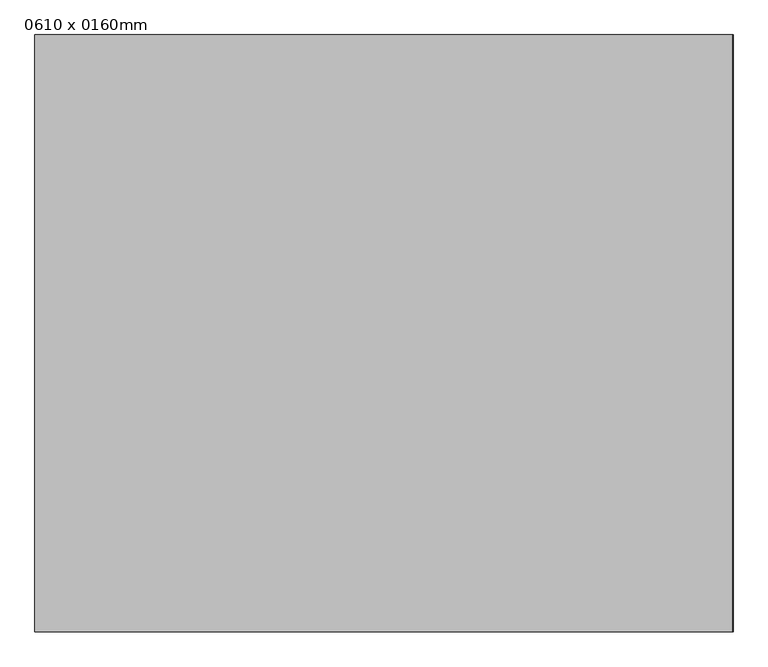
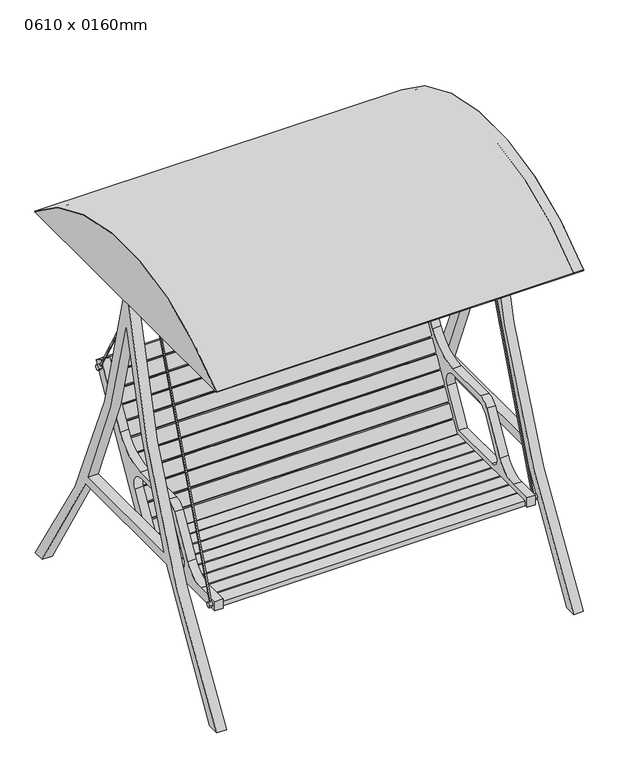
"""IFC4 building model written with IfcOpenShell, lengths in millimetres: furniture geometry, 0610 x 0160mm."""

from ifc_helpers import new_model, si_unit, point, frame, frame_2d, origin, place, context, project, spatial, polyline, circle_curve, trimmed, segment, composite_curve, outline, extrude, source, transform, mapped, element, save


def furniture_0610_x_0160mm_a8fad5e2(model_context):
    return source(origin(), model_context, "Body", "SweptSolid", [
        extrude(outline(composite_curve([segment(trimmed(circle_curve(frame_2d((4189.9023331, 1950.2809332)), 3303.1244251), [point((933.45, 1396.9734505))], [point((1524.0, 0.0))], True, "CARTESIAN"), True, "CONTINUOUS"), segment(polyline([(1524.0, 0.0), (1476.936255, 0.0)]), True, "CONTINUOUS"), segment(trimmed(circle_curve(frame_2d((4189.9023331, 1950.2809332)), 3341.2244251), [point((1476.936255, 0.0))], [point((1186.3373595, 486.5944542))], False, "CARTESIAN"), True, "CONTINUOUS"), segment(polyline([(1186.3373595, 486.5944542), (642.4626405, 486.5944542)]), True, "CONTINUOUS"), segment(trimmed(circle_curve(frame_2d((-2361.1023331, 1950.2809332)), 3341.2244251), [point((642.4626405, 486.5944542))], [point((351.863745, 0.0))], False, "CARTESIAN"), True, "CONTINUOUS"), segment(polyline([(351.863745, 0.0), (304.8, 0.0)]), True, "CONTINUOUS"), segment(trimmed(circle_curve(frame_2d((-2361.1023331, 1950.2809332)), 3303.1244251), [point((304.8, 0.0))], [point((895.35, 1396.9734505))], True, "CARTESIAN"), True, "CONTINUOUS"), segment(polyline([(895.35, 1396.9734505), (895.35, 1524.0), (914.4, 1524.0), (933.45, 1524.0), (933.45, 1396.9734505)]), True, "CONTINUOUS")], self_intersect=False), holes=[composite_curve([segment(polyline([(660.7321842, 524.6944542), (1168.0678158, 524.6944542)]), True, "CONTINUOUS"), segment(trimmed(circle_curve(frame_2d((4189.9023331, 1950.2809332)), 3341.2244251), [point((1168.0678158, 524.6944542))], [point((914.4, 1290.8378915))], False, "CARTESIAN"), True, "CONTINUOUS"), segment(trimmed(circle_curve(frame_2d((-2361.1023331, 1950.2809332)), 3341.2244251), [point((914.4, 1290.8378915))], [point((660.7321842, 524.6944542))], False, "CARTESIAN"), True, "CONTINUOUS")], self_intersect=False)]), frame((-272.362745, 0.0, 0.0), z_axis=(1.0, 0.0, 0.0), x_axis=(0.0, 1.0, 0.0)), (0.0, 0.0, 1.0), 38.1),
        extrude(outline(composite_curve([segment(trimmed(circle_curve(frame_2d((4189.9023331, 1950.2809332)), 3303.1244251), [point((933.45, 1396.9734505))], [point((1524.0, 0.0))], True, "CARTESIAN"), True, "CONTINUOUS"), segment(polyline([(1524.0, 0.0), (1476.936255, 0.0)]), True, "CONTINUOUS"), segment(trimmed(circle_curve(frame_2d((4189.9023331, 1950.2809332)), 3341.2244251), [point((1476.936255, 0.0))], [point((1186.3373595, 486.5944542))], False, "CARTESIAN"), True, "CONTINUOUS"), segment(polyline([(1186.3373595, 486.5944542), (642.4626405, 486.5944542)]), True, "CONTINUOUS"), segment(trimmed(circle_curve(frame_2d((-2361.1023331, 1950.2809332)), 3341.2244251), [point((642.4626405, 486.5944542))], [point((351.863745, 0.0))], False, "CARTESIAN"), True, "CONTINUOUS"), segment(polyline([(351.863745, 0.0), (304.8, 0.0)]), True, "CONTINUOUS"), segment(trimmed(circle_curve(frame_2d((-2361.1023331, 1950.2809332)), 3303.1244251), [point((304.8, 0.0))], [point((895.35, 1396.9734505))], True, "CARTESIAN"), True, "CONTINUOUS"), segment(polyline([(895.35, 1396.9734505), (895.35, 1524.0), (914.4, 1524.0), (933.45, 1524.0), (933.45, 1396.9734505)]), True, "CONTINUOUS")], self_intersect=False), holes=[composite_curve([segment(polyline([(660.7321842, 524.6944542), (1168.0678158, 524.6944542)]), True, "CONTINUOUS"), segment(trimmed(circle_curve(frame_2d((4189.9023331, 1950.2809332)), 3341.2244251), [point((1168.0678158, 524.6944542))], [point((914.4, 1290.8378915))], False, "CARTESIAN"), True, "CONTINUOUS"), segment(trimmed(circle_curve(frame_2d((-2361.1023331, 1950.2809332)), 3341.2244251), [point((914.4, 1290.8378915))], [point((660.7321842, 524.6944542))], False, "CARTESIAN"), True, "CONTINUOUS")], self_intersect=False)]), frame((1111.937255, 0.0, 0.0), z_axis=(1.0, 0.0, 0.0), x_axis=(0.0, 1.0, 0.0)), (0.0, 0.0, 1.0), 38.1),
        extrude(outline(polyline([(1111.937255, 933.45), (1111.937255, 895.35), (-234.262745, 895.35), (-234.262745, 933.45), (1111.937255, 933.45)])), frame((0.0, 0.0, 1484.1023899), z_axis=(0.0, 0.0, 1.0), x_axis=(1.0, 0.0, 0.0)), (0.0, 0.0, 1.0), 39.8976101),
        extrude(outline(composite_curve([segment(trimmed(circle_curve(frame_2d((914.4, 699.3747703)), 926.421113), [point((304.8, 1396.9734505))], [point((1524.0, 1396.9734505))], False, "CARTESIAN"), True, "CONTINUOUS"), segment(polyline([(1524.0, 1396.9734505), (304.8, 1396.9734505)]), True, "CONTINUOUS")], self_intersect=False), holes=[composite_curve([segment(polyline([(376.708681, 1422.3734505), (1452.091319, 1422.3734505)]), True, "CONTINUOUS"), segment(trimmed(circle_curve(frame_2d((914.4, 699.3747703)), 901.021113), [point((1452.091319, 1422.3734505))], [point((376.708681, 1422.3734505))], True, "CARTESIAN"), True, "CONTINUOUS")], self_intersect=False)]), frame((-272.362745, 0.0, 0.0), z_axis=(1.0, 0.0, 0.0), x_axis=(0.0, 1.0, 0.0)), (0.0, 0.0, 1.0), 38.1),
        extrude(outline(composite_curve([segment(trimmed(circle_curve(frame_2d((914.4, 699.3747703)), 926.421113), [point((304.8, 1396.9734505))], [point((1524.0, 1396.9734505))], False, "CARTESIAN"), True, "CONTINUOUS"), segment(polyline([(1524.0, 1396.9734505), (304.8, 1396.9734505)]), True, "CONTINUOUS")], self_intersect=False), holes=[composite_curve([segment(polyline([(376.708681, 1422.3734505), (1452.091319, 1422.3734505)]), True, "CONTINUOUS"), segment(trimmed(circle_curve(frame_2d((914.4, 699.3747703)), 901.021113), [point((1452.091319, 1422.3734505))], [point((376.708681, 1422.3734505))], True, "CARTESIAN"), True, "CONTINUOUS")], self_intersect=False)]), frame((1111.937255, 0.0, 0.0), z_axis=(1.0, 0.0, 0.0), x_axis=(0.0, 1.0, 0.0)), (0.0, 0.0, 1.0), 38.1),
        extrude(outline(composite_curve([segment(trimmed(circle_curve(frame_2d((914.4, 699.3747703)), 926.421113), [point((304.8, 1396.9734505))], [point((1524.0, 1396.9734505))], False, "CARTESIAN"), True, "CONTINUOUS"), segment(polyline([(1524.0, 1396.9734505), (304.8, 1396.9734505)]), True, "CONTINUOUS")], self_intersect=False)), frame((-273.952745, 0.0, 0.0), z_axis=(1.0, 0.0, 0.0), x_axis=(0.0, 1.0, 0.0)), (0.0, 0.0, 1.0), 1.59),
        extrude(outline(composite_curve([segment(trimmed(circle_curve(frame_2d((914.4, 699.3747703)), 926.421113), [point((304.8, 1396.9734505))], [point((1524.0, 1396.9734505))], False, "CARTESIAN"), True, "CONTINUOUS"), segment(polyline([(1524.0, 1396.9734505), (304.8, 1396.9734505)]), True, "CONTINUOUS")], self_intersect=False)), frame((1150.037255, 0.0, 0.0), z_axis=(1.0, 0.0, 0.0), x_axis=(0.0, 1.0, 0.0)), (0.0, 0.0, 1.0), 1.59),
        extrude(outline(composite_curve([segment(trimmed(circle_curve(frame_2d((914.4, 699.3747703)), 926.421113), [point((1524.0, 1396.9734505))], [point((304.8, 1396.9734505))], True, "CARTESIAN"), True, "CONTINUOUS"), segment(polyline([(304.8, 1396.9734505), (304.8, 1399.0836139)]), True, "CONTINUOUS"), segment(trimmed(circle_curve(frame_2d((914.4, 699.3747703)), 928.011113), [point((304.8, 1399.0836139))], [point((1524.0, 1399.0836139))], False, "CARTESIAN"), True, "CONTINUOUS"), segment(polyline([(1524.0, 1399.0836139), (1524.0, 1396.9734505)]), True, "CONTINUOUS")], self_intersect=False)), frame((-273.952745, 0.0, 0.0), z_axis=(1.0, 0.0, 0.0), x_axis=(0.0, 1.0, 0.0)), (0.0, 0.0, 1.0), 1423.99),
        extrude(outline(composite_curve([segment(trimmed(circle_curve(frame_2d((563.6419667, 511.4)), 105.0), [point((563.6419667, 406.4))], [point((654.5746341, 458.9))], True, "CARTESIAN"), True, "CONTINUOUS"), segment(polyline([(654.5746341, 458.9), (741.8122598, 610.0)]), True, "CONTINUOUS"), segment(trimmed(circle_curve(frame_2d((785.11353, 585.0)), 50.0), [point((741.8122598, 610.0))], [point((785.11353, 635.0))], False, "CARTESIAN"), True, "CONTINUOUS"), segment(polyline([(785.11353, 635.0), (968.6699734, 635.0)]), True, "CONTINUOUS"), segment(trimmed(circle_curve(frame_2d((968.6699734, 795.0)), 160.0), [point((968.6699734, 635.0))], [point((1107.2340381, 715.0))], True, "CARTESIAN"), True, "CONTINUOUS"), segment(polyline([(1107.2340381, 715.0), (1233.863745, 934.3290861), (1266.8593129, 915.2790861), (951.0607902, 368.3), (471.863745, 368.3), (471.863745, 406.4), (563.6419667, 406.4)]), True, "CONTINUOUS")], self_intersect=False), holes=[composite_curve([segment(trimmed(circle_curve(frame_2d((807.1413638, 546.8466726)), 62.7533274), [point((807.1413638, 609.6))], [point((752.7953881, 578.2233363))], True, "CARTESIAN"), True, "CONTINUOUS"), segment(polyline([(752.7953881, 578.2233363), (679.5739008, 451.4)]), True, "CONTINUOUS"), segment(trimmed(circle_curve(frame_2d((705.5546629, 436.4)), 30.0), [point((679.5739008, 451.4))], [point((705.5546629, 406.4))], True, "CARTESIAN"), True, "CONTINUOUS"), segment(polyline([(705.5546629, 406.4), (929.063745, 406.4), (1007.4101765, 542.1)]), True, "CONTINUOUS"), segment(trimmed(circle_curve(frame_2d((968.4390333, 564.6)), 45.0), [point((1007.4101765, 542.1))], [point((968.4390333, 609.6))], True, "CARTESIAN"), True, "CONTINUOUS"), segment(polyline([(968.4390333, 609.6), (807.1413638, 609.6)]), True, "CONTINUOUS")], self_intersect=False)]), frame((-184.03019, 0.0, 0.0), z_axis=(1.0, 0.0, 0.0), x_axis=(0.0, 1.0, 0.0)), (0.0, 0.0, 1.0), 32.5713093),
        extrude(outline(composite_curve([segment(trimmed(circle_curve(frame_2d((563.6419667, 511.4)), 105.0), [point((563.6419667, 406.4))], [point((654.5746341, 458.9))], True, "CARTESIAN"), True, "CONTINUOUS"), segment(polyline([(654.5746341, 458.9), (741.8122598, 610.0)]), True, "CONTINUOUS"), segment(trimmed(circle_curve(frame_2d((785.11353, 585.0)), 50.0), [point((741.8122598, 610.0))], [point((785.11353, 635.0))], False, "CARTESIAN"), True, "CONTINUOUS"), segment(polyline([(785.11353, 635.0), (968.6699734, 635.0)]), True, "CONTINUOUS"), segment(trimmed(circle_curve(frame_2d((968.6699734, 795.0)), 160.0), [point((968.6699734, 635.0))], [point((1107.2340381, 715.0))], True, "CARTESIAN"), True, "CONTINUOUS"), segment(polyline([(1107.2340381, 715.0), (1233.863745, 934.3290861), (1266.8593129, 915.2790861), (951.0607902, 368.3), (471.863745, 368.3), (471.863745, 406.4), (563.6419667, 406.4)]), True, "CONTINUOUS")], self_intersect=False), holes=[composite_curve([segment(trimmed(circle_curve(frame_2d((807.1413638, 546.8466726)), 62.7533274), [point((807.1413638, 609.6))], [point((752.7953881, 578.2233363))], True, "CARTESIAN"), True, "CONTINUOUS"), segment(polyline([(752.7953881, 578.2233363), (679.5739008, 451.4)]), True, "CONTINUOUS"), segment(trimmed(circle_curve(frame_2d((705.5546629, 436.4)), 30.0), [point((679.5739008, 451.4))], [point((705.5546629, 406.4))], True, "CARTESIAN"), True, "CONTINUOUS"), segment(polyline([(705.5546629, 406.4), (929.063745, 406.4), (1007.4101765, 542.1)]), True, "CONTINUOUS"), segment(trimmed(circle_curve(frame_2d((968.4390333, 564.6)), 45.0), [point((1007.4101765, 542.1))], [point((968.4390333, 609.6))], True, "CARTESIAN"), True, "CONTINUOUS"), segment(polyline([(968.4390333, 609.6), (807.1413638, 609.6)]), True, "CONTINUOUS")], self_intersect=False)]), frame((1027.5433908, 0.0, 0.0), z_axis=(1.0, 0.0, 0.0), x_axis=(0.0, 1.0, 0.0)), (0.0, 0.0, 1.0), 32.5713093),
        extrude(outline(polyline([(0.0, -19.0500001), (0.0, 0.0), (1179.0022715, 0.0), (1179.0022715, -19.0500001), (0.0, -19.0500001)])), frame((1027.5433908, 1224.9615289, 880.8099956), z_axis=(0.0, 0.5000000000000067, 0.8660254037844349), x_axis=(-1.0, 0.0, 0.0)), (0.0, 0.0, 1.0), 50.8),
        extrude(outline(polyline([(0.0, -19.0500001), (0.0, 0.0), (1179.0022715, 0.0), (1179.0022715, -19.0500001), (0.0, -19.0500001)])), frame((1027.5433908, 1196.3865289, 831.3166438), z_axis=(0.0, 0.5000000000000067, 0.8660254037844349), x_axis=(-1.0, 0.0, 0.0)), (0.0, 0.0, 1.0), 50.8),
        extrude(outline(polyline([(0.0, -19.0500001), (0.0, 0.0), (1179.0022715, 0.0), (1179.0022715, -19.0500001), (0.0, -19.0500001)])), frame((1027.5433908, 1167.8115289, 781.823292), z_axis=(0.0, 0.5000000000000067, 0.8660254037844349), x_axis=(-1.0, 0.0, 0.0)), (0.0, 0.0, 1.0), 50.8),
        extrude(outline(polyline([(0.0, -19.0500001), (0.0, 0.0), (1179.0022715, 0.0), (1179.0022715, -19.0500001), (0.0, -19.0500001)])), frame((1027.5433908, 1139.2365289, 732.3299402), z_axis=(0.0, 0.5000000000000067, 0.8660254037844349), x_axis=(-1.0, 0.0, 0.0)), (0.0, 0.0, 1.0), 50.8),
        extrude(outline(polyline([(0.0, -19.0500001), (0.0, 0.0), (1179.0022715, 0.0), (1179.0022715, -19.0500001), (0.0, -19.0500001)])), frame((1027.5433908, 1110.6615289, 682.8365883), z_axis=(0.0, 0.5000000000000067, 0.8660254037844349), x_axis=(-1.0, 0.0, 0.0)), (0.0, 0.0, 1.0), 50.8),
        extrude(outline(polyline([(0.0, -19.0500001), (0.0, 0.0), (1179.0022715, 0.0), (1179.0022715, -19.0500001), (0.0, -19.0500001)])), frame((1027.5433908, 1082.0865289, 633.3432365), z_axis=(0.0, 0.5000000000000067, 0.8660254037844349), x_axis=(-1.0, 0.0, 0.0)), (0.0, 0.0, 1.0), 50.8),
        extrude(outline(polyline([(0.0, -19.0500001), (0.0, 0.0), (1179.0022715, 0.0), (1179.0022715, -19.0500001), (0.0, -19.0500001)])), frame((1027.5433908, 1053.5115289, 583.8498847), z_axis=(0.0, 0.5000000000000067, 0.8660254037844349), x_axis=(-1.0, 0.0, 0.0)), (0.0, 0.0, 1.0), 50.8),
        extrude(outline(polyline([(0.0, -19.0500001), (0.0, 0.0), (1179.0022715, 0.0), (1179.0022715, -19.0500001), (0.0, -19.0500001)])), frame((1027.5433908, 1024.9365289, 534.3565329), z_axis=(0.0, 0.5000000000000067, 0.8660254037844349), x_axis=(-1.0, 0.0, 0.0)), (0.0, 0.0, 1.0), 50.8),
        extrude(outline(polyline([(0.0, -19.0500001), (0.0, 0.0), (1179.0022715, 0.0), (1179.0022715, -19.0500001), (0.0, -19.0500001)])), frame((1027.5433908, 996.3615289, 484.863181), z_axis=(0.0, 0.5000000000000067, 0.8660254037844349), x_axis=(-1.0, 0.0, 0.0)), (0.0, 0.0, 1.0), 50.8),
        extrude(outline(polyline([(0.0, -19.0500001), (0.0, 0.0), (1179.0022715, 0.0), (1179.0022715, -19.0500001), (0.0, -19.0500001)])), frame((1027.5433908, 967.7865289, 435.3698292), z_axis=(0.0, 0.5000000000000067, 0.8660254037844349), x_axis=(-1.0, 0.0, 0.0)), (0.0, 0.0, 1.0), 50.8),
        extrude(outline(polyline([(0.0, -19.0500001), (0.0, 0.0), (1179.0022715, 0.0), (1179.0022715, -19.0500001), (0.0, -19.0500001)])), frame((1027.5433908, 939.2115289, 385.8764774), z_axis=(0.0, 0.5000000000000067, 0.8660254037844349), x_axis=(-1.0, 0.0, 0.0)), (0.0, 0.0, 1.0), 50.8),
        extrude(outline(polyline([(1027.5433908, 933.8211), (1027.5433908, 883.0211), (-151.4588807, 883.0211), (-151.4588807, 933.8211), (1027.5433908, 933.8211)])), frame((0.0, 0.0, 368.3), z_axis=(0.0, 0.0, 1.0), x_axis=(1.0, 0.0, 0.0)), (0.0, 0.0, 1.0), 19.05),
        extrude(outline(polyline([(1027.5433908, 876.6711), (1027.5433908, 825.8711), (-151.4588807, 825.8711), (-151.4588807, 876.6711), (1027.5433908, 876.6711)])), frame((0.0, 0.0, 368.3), z_axis=(0.0, 0.0, 1.0), x_axis=(1.0, 0.0, 0.0)), (0.0, 0.0, 1.0), 19.05),
        extrude(outline(polyline([(1027.5433908, 819.5211), (1027.5433908, 768.7211), (-151.4588807, 768.7211), (-151.4588807, 819.5211), (1027.5433908, 819.5211)])), frame((0.0, 0.0, 368.3), z_axis=(0.0, 0.0, 1.0), x_axis=(1.0, 0.0, 0.0)), (0.0, 0.0, 1.0), 19.05),
        extrude(outline(polyline([(1027.5433908, 762.3711), (1027.5433908, 711.5711), (-151.4588807, 711.5711), (-151.4588807, 762.3711), (1027.5433908, 762.3711)])), frame((0.0, 0.0, 368.3), z_axis=(0.0, 0.0, 1.0), x_axis=(1.0, 0.0, 0.0)), (0.0, 0.0, 1.0), 19.05),
        extrude(outline(polyline([(1027.5433908, 705.2211), (1027.5433908, 654.4211), (-151.4588807, 654.4211), (-151.4588807, 705.2211), (1027.5433908, 705.2211)])), frame((0.0, 0.0, 368.3), z_axis=(0.0, 0.0, 1.0), x_axis=(1.0, 0.0, 0.0)), (0.0, 0.0, 1.0), 19.05),
        extrude(outline(polyline([(1027.5433908, 648.0711), (1027.5433908, 597.2711), (-151.4588807, 597.2711), (-151.4588807, 648.0711), (1027.5433908, 648.0711)])), frame((0.0, 0.0, 368.3), z_axis=(0.0, 0.0, 1.0), x_axis=(1.0, 0.0, 0.0)), (0.0, 0.0, 1.0), 19.05),
        extrude(outline(polyline([(1027.5433908, 590.9211), (1027.5433908, 540.1211), (-151.4588807, 540.1211), (-151.4588807, 590.9211), (1027.5433908, 590.9211)])), frame((0.0, 0.0, 368.3), z_axis=(0.0, 0.0, 1.0), x_axis=(1.0, 0.0, 0.0)), (0.0, 0.0, 1.0), 19.05),
        extrude(outline(polyline([(1027.5433908, 533.7711), (1027.5433908, 482.9711), (-151.4588807, 482.9711), (-151.4588807, 533.7711), (1027.5433908, 533.7711)])), frame((0.0, 0.0, 368.3), z_axis=(0.0, 0.0, 1.0), x_axis=(1.0, 0.0, 0.0)), (0.0, 0.0, 1.0), 19.05),
        extrude(outline(polyline([(914.4, 1484.1023899), (1241.1891484, 905.4891111), (1236.3748088, 902.7700689), (911.842017, 1477.3882398), (494.9813942, 383.2195737), (489.4362629, 385.3321793), (908.05, 1484.1023899), (914.4, 1484.1023899)])), frame((-188.7825876, 0.0, 0.0), z_axis=(1.0, 0.0, 0.0), x_axis=(0.0, 1.0, 0.0)), (0.0, 0.0, 1.0), 4.7523976),
        extrude(outline(composite_curve([segment(trimmed(circle_curve(frame_2d((1238.7819786, 904.12959)), 10.0), [point((1228.7819786, 904.12959))], [point((1248.7819786, 904.12959))], False, "CARTESIAN"), True, "CONTINUOUS"), segment(trimmed(circle_curve(frame_2d((1238.7819786, 904.12959)), 10.0), [point((1248.7819786, 904.12959))], [point((1228.7819786, 904.12959))], False, "CARTESIAN"), True, "CONTINUOUS")], self_intersect=False)), frame((-196.8218142, 0.0, 0.0), z_axis=(1.0, 0.0, 0.0), x_axis=(0.0, 1.0, 0.0)), (0.0, 0.0, 1.0), 12.7916242),
        extrude(outline(composite_curve([segment(trimmed(circle_curve(frame_2d((492.2088285, 384.2758765)), 10.0), [point((482.2088285, 384.2758765))], [point((502.2088285, 384.2758765))], False, "CARTESIAN"), True, "CONTINUOUS"), segment(trimmed(circle_curve(frame_2d((492.2088285, 384.2758765)), 10.0), [point((502.2088285, 384.2758765))], [point((482.2088285, 384.2758765))], False, "CARTESIAN"), True, "CONTINUOUS")], self_intersect=False)), frame((-196.8218142, 0.0, 0.0), z_axis=(1.0, 0.0, 0.0), x_axis=(0.0, 1.0, 0.0)), (0.0, 0.0, 1.0), 12.7916242),
        extrude(outline(polyline([(914.4, 1484.1023899), (1241.1891484, 905.4891111), (1236.3748088, 902.7700689), (911.842017, 1477.3882398), (494.9813942, 383.2195737), (489.4362629, 385.3321793), (908.05, 1484.1023899), (914.4, 1484.1023899)])), frame((1061.7047, 0.0, 0.0), z_axis=(1.0, 0.0, 0.0), x_axis=(0.0, 1.0, 0.0)), (0.0, 0.0, 1.0), 4.7523976),
        extrude(outline(composite_curve([segment(trimmed(circle_curve(frame_2d((1238.7819786, 904.12959)), 10.0), [point((1228.7819786, 904.12959))], [point((1248.7819786, 904.12959))], False, "CARTESIAN"), True, "CONTINUOUS"), segment(trimmed(circle_curve(frame_2d((1238.7819786, 904.12959)), 10.0), [point((1248.7819786, 904.12959))], [point((1228.7819786, 904.12959))], False, "CARTESIAN"), True, "CONTINUOUS")], self_intersect=False)), frame((1061.7047, 0.0, 0.0), z_axis=(1.0, 0.0, 0.0), x_axis=(0.0, 1.0, 0.0)), (0.0, 0.0, 1.0), 12.7916242),
        extrude(outline(composite_curve([segment(trimmed(circle_curve(frame_2d((492.2088285, 384.2758765)), 10.0), [point((482.2088285, 384.2758765))], [point((502.2088285, 384.2758765))], False, "CARTESIAN"), True, "CONTINUOUS"), segment(trimmed(circle_curve(frame_2d((492.2088285, 384.2758765)), 10.0), [point((502.2088285, 384.2758765))], [point((482.2088285, 384.2758765))], False, "CARTESIAN"), True, "CONTINUOUS")], self_intersect=False)), frame((1061.7047, 0.0, 0.0), z_axis=(1.0, 0.0, 0.0), x_axis=(0.0, 1.0, 0.0)), (0.0, 0.0, 1.0), 12.7916242),
    ])


if __name__ == "__main__":
    model = new_model("IFC4")
    model_context = context("Model", 3, world=origin())
    ifc_project = project(units=[si_unit("LENGTHUNIT", "METRE", prefix="MILLI")], contexts=[model_context])
    site = spatial("IfcSite", under=ifc_project)
    building = spatial("IfcBuilding", under=site)
    placement = place(None, origin())
    furniture_0610_x_0160mm_shape = furniture_0610_x_0160mm_a8fad5e2(model_context)
    element("IfcFurniture", 1, ObjectType="0610 x 0160mm", at=placement, inside=building, context=model_context, shape_type="MappedRepresentation", body=[
        mapped(furniture_0610_x_0160mm_shape, transform((0.0, 0.0, 0.0), x_axis=(1.0, 0.0, 0.0), y_axis=(0.0, 1.0, 0.0), z_axis=(0.0, 0.0, 1.0))),
    ])
    save(model, "model.ifc")

# Revit data of these elements
# Type "0610 x 0160mm"
#   Height = 2' - 6"
#   Length = 2' - 0.01575"
#   Width = 2' - 0.01575"
#   Base Material = Wood - Birch
#   Top Material = Laminate - Ivory, Matte
#   Default Elevation = 0
# Element 1 (IfcFurniture, "0610 x 0160mm")
#   Materials on its faces: "wood finish", "steel", "Laminate - Ivory, Matte", "fabric"
# Materials
#   "Wood - Birch": class "Metal", colour RGB 105 77 58, transparency 0
#   "Laminate - Ivory, Matte": colour RGB 247 247 239, transparency 0
#   "wood finish": class "Generic", colour RGB 120 120 120, transparency 0, Cost = 0
#   "steel": class "Generic", colour RGB 120 120 120, transparency 0, Cost = 0
#   "fabric": class "Fabric", colour RGB 198 193 133, transparency 0
